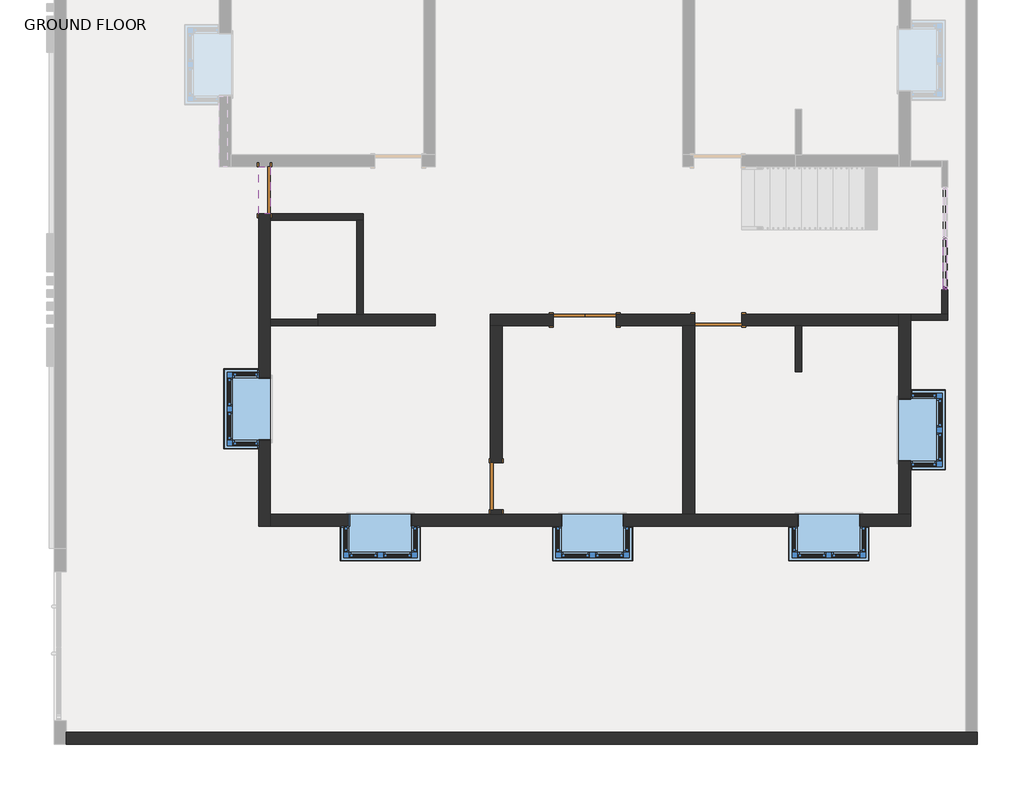
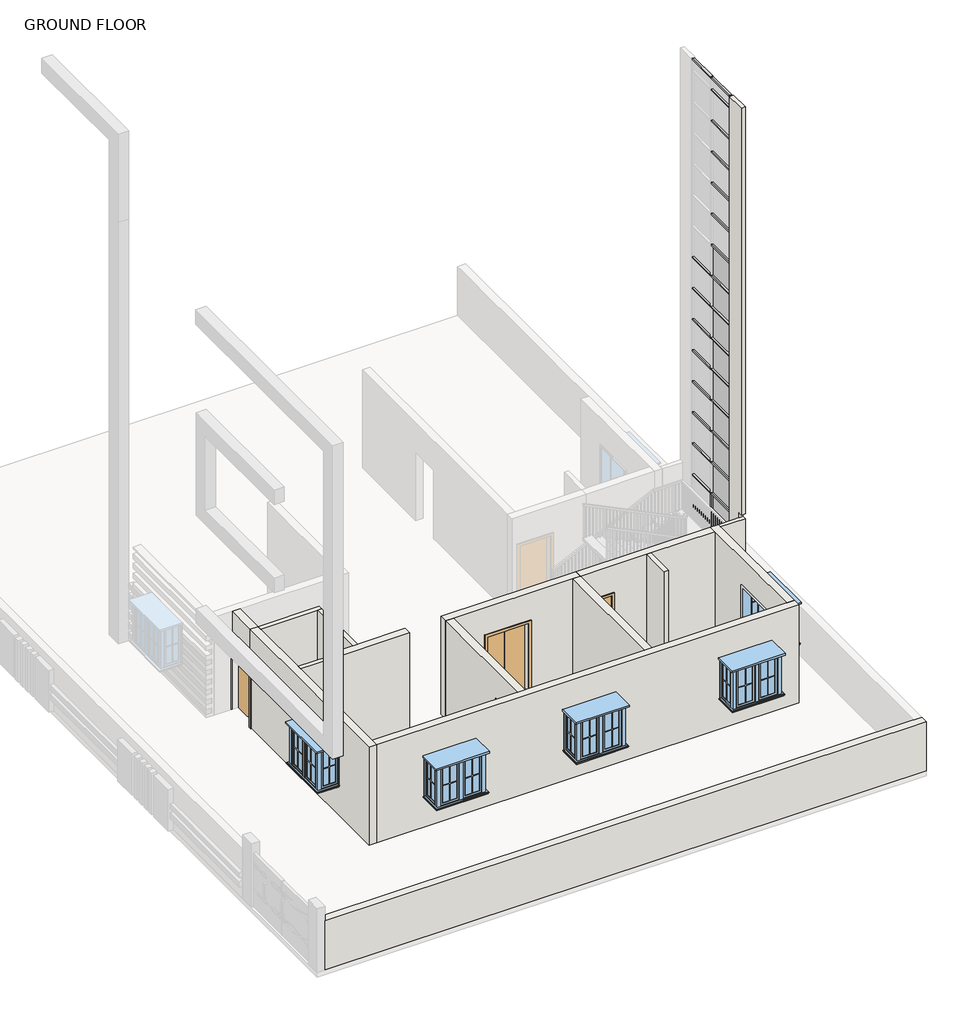
# One storey, part 1 of 5: 66 members, 16 walls, 11 plates, 5 windows, 4 doors.
"""IFC4 building model written with IfcOpenShell, lengths in millimetres."""

from ifc_helpers import new_model, si_unit, frame, origin, origin_with_axes, place, context, project, spatial, polyline, outline, extrude, faceted_brep, transform, mapped, element, save
from components import door_double_flush_panel_4_x7_7c704b5a, door_a90ba1ad, door_0ca8825f, member_c65a811d, member_51048147, member_2967a2d8, member_1ede677d, member_eea045b6, member_e7145701, member_32999801, member_18929904, system_panel_glazed_7f04015b, window_bay_casement_box_90_degree_angle_4_x4_x2_07b705a1

model = new_model("IFC4")

# Units and contexts
model_context = context("Model", 3, world=origin())
ifc_project = project(units=[si_unit("LENGTHUNIT", "METRE", prefix="MILLI")], contexts=[model_context])

# Site, building, storey
site = spatial("IfcSite", under=ifc_project)
building = spatial("IfcBuilding", under=site)
storey = spatial("IfcBuildingStorey", under=building, Name="GROUND FLOOR", Elevation=0.0)

# Doors
placement = place(None, origin())
door_double_flush_panel_4_x7_shape = door_double_flush_panel_4_x7_7c704b5a(model_context)
element("IfcDoor", 1, ObjectType="Door-Double-Flush_Panel : 4'x7'", at=placement, inside=storey, context=model_context, shape_type="MappedRepresentation", body=[
    mapped(door_double_flush_panel_4_x7_shape, transform((78.2584916, -2751.066654, 0.0), x_axis=(1.0, 0.0, 0.0), y_axis=(0.0, 1.0, 0.0), z_axis=(0.0, 0.0, 1.0))),
])
door_shape = door_a90ba1ad(model_context)
element("IfcDoor", 2, ObjectType="Single-Flush : 36\" x 84\"", at=placement, inside=storey, context=model_context, shape_type="MappedRepresentation", body=[
    mapped(door_shape, transform((-1636.2415084, -5976.866654, 0.0), x_axis=(0.0, -1.0, 0.0), y_axis=(1.0, 0.0, 0.0), z_axis=(0.0, 0.0, 1.0))),
])
door_2_shape = door_0ca8825f(model_context)
element("IfcDoor", 3, ObjectType="Single-Flush : 36\" x 84\"", at=placement, inside=storey, context=model_context, shape_type="MappedRepresentation", body=[
    mapped(door_2_shape, transform((2669.0584916, -2751.066654, 0.0), x_axis=(-1.0, 0.0, 0.0), y_axis=(0.0, -1.0, 0.0), z_axis=(0.0, 0.0, 1.0))),
])
element("IfcDoor", 4, ObjectType="Single-Flush : 36\" x 84\"", at=placement, inside=storey, context=model_context, shape_type="MappedRepresentation", body=[
    mapped(door_2_shape, transform((-6132.0415084, -236.466654, 0.0), x_axis=(0.0, -1.0, 0.0), y_axis=(1.0, 0.0, 0.0), z_axis=(0.0, 0.0, 1.0))),
])

# Members
member_shape = member_c65a811d(model_context)
element("IfcMember", 5, ObjectType="Rectangular Mullion : 1.5\" x 2.5\" rectangular", at=placement, inside=storey, context=model_context, shape_type="MappedRepresentation", body=[
    mapped(member_shape, transform((7067.5550459, -1147.0566543, 15849.6), x_axis=(0.0, 0.0, 1.0), y_axis=(-1.0, 0.0, 0.0), z_axis=(0.0, -1.0, 0.0))),
])
element("IfcMember", 6, ObjectType="Rectangular Mullion : 1.5\" x 2.5\" rectangular", at=placement, inside=storey, context=model_context, shape_type="MappedRepresentation", body=[
    mapped(member_shape, transform((7067.5550459, -2112.2566543, 15849.6), x_axis=(0.0, 0.0, 1.0), y_axis=(-1.0, 0.0, 0.0), z_axis=(0.0, -1.0, 0.0))),
])
element("IfcMember", 7, ObjectType="Rectangular Mullion : 1.5\" x 2.5\" rectangular", at=placement, inside=storey, context=model_context, shape_type="MappedRepresentation", body=[
    mapped(member_shape, transform((7067.5550459, -1185.1566543, 0.0), x_axis=(0.0, 0.0, -1.0), y_axis=(-1.0, 0.0, 0.0), z_axis=(0.0, 1.0, 0.0))),
])
member_2_shape = member_51048147(model_context)
element("IfcMember", 8, ObjectType="Rectangular Mullion : 1.5\" x 2.5\" rectangular", at=placement, inside=storey, context=model_context, shape_type="MappedRepresentation", body=[
    mapped(member_2_shape, transform((7067.5550459, -1147.0566543, 984.25), x_axis=(0.0, 0.0, 1.0), y_axis=(-1.0, 0.0, 0.0), z_axis=(0.0, -1.0, 0.0))),
])
element("IfcMember", 9, ObjectType="Rectangular Mullion : 1.5\" x 2.5\" rectangular", at=placement, inside=storey, context=model_context, shape_type="MappedRepresentation", body=[
    mapped(member_2_shape, transform((7067.5550459, -2112.2566543, 984.25), x_axis=(0.0, 0.0, 1.0), y_axis=(-1.0, 0.0, 0.0), z_axis=(0.0, -1.0, 0.0))),
])
element("IfcMember", 10, ObjectType="Rectangular Mullion : 1.5\" x 2.5\" rectangular", at=placement, inside=storey, context=model_context, shape_type="MappedRepresentation", body=[
    mapped(member_2_shape, transform((7067.5550459, -1147.0566543, 1949.45), x_axis=(0.0, 0.0, 1.0), y_axis=(-1.0, 0.0, 0.0), z_axis=(0.0, -1.0, 0.0))),
])
element("IfcMember", 11, ObjectType="Rectangular Mullion : 1.5\" x 2.5\" rectangular", at=placement, inside=storey, context=model_context, shape_type="MappedRepresentation", body=[
    mapped(member_2_shape, transform((7067.5550459, -2112.2566543, 1949.45), x_axis=(0.0, 0.0, 1.0), y_axis=(-1.0, 0.0, 0.0), z_axis=(0.0, -1.0, 0.0))),
])
element("IfcMember", 12, ObjectType="Rectangular Mullion : 1.5\" x 2.5\" rectangular", at=placement, inside=storey, context=model_context, shape_type="MappedRepresentation", body=[
    mapped(member_2_shape, transform((7067.5550459, -1147.0566543, 2914.65), x_axis=(0.0, 0.0, 1.0), y_axis=(-1.0, 0.0, 0.0), z_axis=(0.0, -1.0, 0.0))),
])
element("IfcMember", 13, ObjectType="Rectangular Mullion : 1.5\" x 2.5\" rectangular", at=placement, inside=storey, context=model_context, shape_type="MappedRepresentation", body=[
    mapped(member_2_shape, transform((7067.5550459, -2112.2566543, 2914.65), x_axis=(0.0, 0.0, 1.0), y_axis=(-1.0, 0.0, 0.0), z_axis=(0.0, -1.0, 0.0))),
])
element("IfcMember", 14, ObjectType="Rectangular Mullion : 1.5\" x 2.5\" rectangular", at=placement, inside=storey, context=model_context, shape_type="MappedRepresentation", body=[
    mapped(member_2_shape, transform((7067.5550459, -1147.0566543, 3879.85), x_axis=(0.0, 0.0, 1.0), y_axis=(-1.0, 0.0, 0.0), z_axis=(0.0, -1.0, 0.0))),
])
element("IfcMember", 15, ObjectType="Rectangular Mullion : 1.5\" x 2.5\" rectangular", at=placement, inside=storey, context=model_context, shape_type="MappedRepresentation", body=[
    mapped(member_2_shape, transform((7067.5550459, -2112.2566543, 3879.85), x_axis=(0.0, 0.0, 1.0), y_axis=(-1.0, 0.0, 0.0), z_axis=(0.0, -1.0, 0.0))),
])
element("IfcMember", 16, ObjectType="Rectangular Mullion : 1.5\" x 2.5\" rectangular", at=placement, inside=storey, context=model_context, shape_type="MappedRepresentation", body=[
    mapped(member_2_shape, transform((7067.5550459, -1147.0566543, 4845.05), x_axis=(0.0, 0.0, 1.0), y_axis=(-1.0, 0.0, 0.0), z_axis=(0.0, -1.0, 0.0))),
])
element("IfcMember", 17, ObjectType="Rectangular Mullion : 1.5\" x 2.5\" rectangular", at=placement, inside=storey, context=model_context, shape_type="MappedRepresentation", body=[
    mapped(member_2_shape, transform((7067.5550459, -2112.2566543, 4845.05), x_axis=(0.0, 0.0, 1.0), y_axis=(-1.0, 0.0, 0.0), z_axis=(0.0, -1.0, 0.0))),
])
element("IfcMember", 18, ObjectType="Rectangular Mullion : 1.5\" x 2.5\" rectangular", at=placement, inside=storey, context=model_context, shape_type="MappedRepresentation", body=[
    mapped(member_2_shape, transform((7067.5550459, -1147.0566543, 5810.25), x_axis=(0.0, 0.0, 1.0), y_axis=(-1.0, 0.0, 0.0), z_axis=(0.0, -1.0, 0.0))),
])
element("IfcMember", 19, ObjectType="Rectangular Mullion : 1.5\" x 2.5\" rectangular", at=placement, inside=storey, context=model_context, shape_type="MappedRepresentation", body=[
    mapped(member_2_shape, transform((7067.5550459, -2112.2566543, 5810.25), x_axis=(0.0, 0.0, 1.0), y_axis=(-1.0, 0.0, 0.0), z_axis=(0.0, -1.0, 0.0))),
])
element("IfcMember", 20, ObjectType="Rectangular Mullion : 1.5\" x 2.5\" rectangular", at=placement, inside=storey, context=model_context, shape_type="MappedRepresentation", body=[
    mapped(member_2_shape, transform((7067.5550459, -1147.0566543, 6775.45), x_axis=(0.0, 0.0, 1.0), y_axis=(-1.0, 0.0, 0.0), z_axis=(0.0, -1.0, 0.0))),
])
element("IfcMember", 21, ObjectType="Rectangular Mullion : 1.5\" x 2.5\" rectangular", at=placement, inside=storey, context=model_context, shape_type="MappedRepresentation", body=[
    mapped(member_2_shape, transform((7067.5550459, -2112.2566543, 6775.45), x_axis=(0.0, 0.0, 1.0), y_axis=(-1.0, 0.0, 0.0), z_axis=(0.0, -1.0, 0.0))),
])
element("IfcMember", 22, ObjectType="Rectangular Mullion : 1.5\" x 2.5\" rectangular", at=placement, inside=storey, context=model_context, shape_type="MappedRepresentation", body=[
    mapped(member_2_shape, transform((7067.5550459, -1147.0566543, 7740.65), x_axis=(0.0, 0.0, 1.0), y_axis=(-1.0, 0.0, 0.0), z_axis=(0.0, -1.0, 0.0))),
])
element("IfcMember", 23, ObjectType="Rectangular Mullion : 1.5\" x 2.5\" rectangular", at=placement, inside=storey, context=model_context, shape_type="MappedRepresentation", body=[
    mapped(member_2_shape, transform((7067.5550459, -2112.2566543, 7740.65), x_axis=(0.0, 0.0, 1.0), y_axis=(-1.0, 0.0, 0.0), z_axis=(0.0, -1.0, 0.0))),
])
element("IfcMember", 24, ObjectType="Rectangular Mullion : 1.5\" x 2.5\" rectangular", at=placement, inside=storey, context=model_context, shape_type="MappedRepresentation", body=[
    mapped(member_2_shape, transform((7067.5550459, -1147.0566543, 8705.85), x_axis=(0.0, 0.0, 1.0), y_axis=(-1.0, 0.0, 0.0), z_axis=(0.0, -1.0, 0.0))),
])
element("IfcMember", 25, ObjectType="Rectangular Mullion : 1.5\" x 2.5\" rectangular", at=placement, inside=storey, context=model_context, shape_type="MappedRepresentation", body=[
    mapped(member_2_shape, transform((7067.5550459, -2112.2566543, 8705.85), x_axis=(0.0, 0.0, 1.0), y_axis=(-1.0, 0.0, 0.0), z_axis=(0.0, -1.0, 0.0))),
])
element("IfcMember", 26, ObjectType="Rectangular Mullion : 1.5\" x 2.5\" rectangular", at=placement, inside=storey, context=model_context, shape_type="MappedRepresentation", body=[
    mapped(member_2_shape, transform((7067.5550459, -1147.0566543, 9671.05), x_axis=(0.0, 0.0, 1.0), y_axis=(-1.0, 0.0, 0.0), z_axis=(0.0, -1.0, 0.0))),
])
element("IfcMember", 27, ObjectType="Rectangular Mullion : 1.5\" x 2.5\" rectangular", at=placement, inside=storey, context=model_context, shape_type="MappedRepresentation", body=[
    mapped(member_2_shape, transform((7067.5550459, -2112.2566543, 9671.05), x_axis=(0.0, 0.0, 1.0), y_axis=(-1.0, 0.0, 0.0), z_axis=(0.0, -1.0, 0.0))),
])
element("IfcMember", 28, ObjectType="Rectangular Mullion : 1.5\" x 2.5\" rectangular", at=placement, inside=storey, context=model_context, shape_type="MappedRepresentation", body=[
    mapped(member_2_shape, transform((7067.5550459, -2112.2566543, 10636.25), x_axis=(0.0, 0.0, 1.0), y_axis=(-1.0, 0.0, 0.0), z_axis=(0.0, -1.0, 0.0))),
])
element("IfcMember", 29, ObjectType="Rectangular Mullion : 1.5\" x 2.5\" rectangular", at=placement, inside=storey, context=model_context, shape_type="MappedRepresentation", body=[
    mapped(member_2_shape, transform((7067.5550459, -2112.2566543, 11601.45), x_axis=(0.0, 0.0, 1.0), y_axis=(-1.0, 0.0, 0.0), z_axis=(0.0, -1.0, 0.0))),
])
element("IfcMember", 30, ObjectType="Rectangular Mullion : 1.5\" x 2.5\" rectangular", at=placement, inside=storey, context=model_context, shape_type="MappedRepresentation", body=[
    mapped(member_2_shape, transform((7067.5550459, -2112.2566543, 12566.65), x_axis=(0.0, 0.0, 1.0), y_axis=(-1.0, 0.0, 0.0), z_axis=(0.0, -1.0, 0.0))),
])
element("IfcMember", 31, ObjectType="Rectangular Mullion : 1.5\" x 2.5\" rectangular", at=placement, inside=storey, context=model_context, shape_type="MappedRepresentation", body=[
    mapped(member_2_shape, transform((7067.5550459, -2112.2566543, 13531.85), x_axis=(0.0, 0.0, 1.0), y_axis=(-1.0, 0.0, 0.0), z_axis=(0.0, -1.0, 0.0))),
])
element("IfcMember", 32, ObjectType="Rectangular Mullion : 1.5\" x 2.5\" rectangular", at=placement, inside=storey, context=model_context, shape_type="MappedRepresentation", body=[
    mapped(member_2_shape, transform((7067.5550459, -2112.2566543, 14497.05), x_axis=(0.0, 0.0, 1.0), y_axis=(-1.0, 0.0, 0.0), z_axis=(0.0, -1.0, 0.0))),
])
element("IfcMember", 33, ObjectType="Rectangular Mullion : 1.5\" x 2.5\" rectangular", at=placement, inside=storey, context=model_context, shape_type="MappedRepresentation", body=[
    mapped(member_2_shape, transform((7067.5550459, -2112.2566543, 15462.25), x_axis=(0.0, 0.0, 1.0), y_axis=(-1.0, 0.0, 0.0), z_axis=(0.0, -1.0, 0.0))),
])
member_3_shape = member_2967a2d8(model_context)
element("IfcMember", 34, ObjectType="Rectangular Mullion : 1.5\" x 2.5\" rectangular", at=placement, inside=storey, context=model_context, shape_type="MappedRepresentation", body=[
    mapped(member_3_shape, transform((7067.5550459, -1166.1066543, 0.0), x_axis=(0.0, -1.0, 0.0), y_axis=(-1.0, 0.0, 0.0), z_axis=(0.0, 0.0, -1.0))),
])
element("IfcMember", 35, ObjectType="Rectangular Mullion : 1.5\" x 2.5\" rectangular", at=placement, inside=storey, context=model_context, shape_type="MappedRepresentation", body=[
    mapped(member_3_shape, transform((7067.5550459, -2131.3066543, 0.0), x_axis=(0.0, -1.0, 0.0), y_axis=(-1.0, 0.0, 0.0), z_axis=(0.0, 0.0, -1.0))),
])
member_4_shape = member_1ede677d(model_context)
element("IfcMember", 36, ObjectType="Rectangular Mullion : 1.5\" x 2.5\" rectangular", at=placement, inside=storey, context=model_context, shape_type="MappedRepresentation", body=[
    mapped(member_4_shape, transform((7067.5550459, -1166.1066543, 984.25), x_axis=(0.0, -1.0, 0.0), y_axis=(-1.0, 0.0, 0.0), z_axis=(0.0, 0.0, -1.0))),
])
element("IfcMember", 37, ObjectType="Rectangular Mullion : 1.5\" x 2.5\" rectangular", at=placement, inside=storey, context=model_context, shape_type="MappedRepresentation", body=[
    mapped(member_4_shape, transform((7067.5550459, -1166.1066543, 1949.45), x_axis=(0.0, -1.0, 0.0), y_axis=(-1.0, 0.0, 0.0), z_axis=(0.0, 0.0, -1.0))),
])
element("IfcMember", 38, ObjectType="Rectangular Mullion : 1.5\" x 2.5\" rectangular", at=placement, inside=storey, context=model_context, shape_type="MappedRepresentation", body=[
    mapped(member_4_shape, transform((7067.5550459, -2131.3066543, 984.25), x_axis=(0.0, -1.0, 0.0), y_axis=(-1.0, 0.0, 0.0), z_axis=(0.0, 0.0, -1.0))),
])
element("IfcMember", 39, ObjectType="Rectangular Mullion : 1.5\" x 2.5\" rectangular", at=placement, inside=storey, context=model_context, shape_type="MappedRepresentation", body=[
    mapped(member_4_shape, transform((7067.5550459, -2131.3066543, 1949.45), x_axis=(0.0, -1.0, 0.0), y_axis=(-1.0, 0.0, 0.0), z_axis=(0.0, 0.0, -1.0))),
])
element("IfcMember", 40, ObjectType="Rectangular Mullion : 1.5\" x 2.5\" rectangular", at=placement, inside=storey, context=model_context, shape_type="MappedRepresentation", body=[
    mapped(member_4_shape, transform((7067.5550459, -2131.3066543, 2914.65), x_axis=(0.0, -1.0, 0.0), y_axis=(-1.0, 0.0, 0.0), z_axis=(0.0, 0.0, -1.0))),
])
element("IfcMember", 41, ObjectType="Rectangular Mullion : 1.5\" x 2.5\" rectangular", at=placement, inside=storey, context=model_context, shape_type="MappedRepresentation", body=[
    mapped(member_4_shape, transform((7067.5550459, -2131.3066543, 3879.85), x_axis=(0.0, -1.0, 0.0), y_axis=(-1.0, 0.0, 0.0), z_axis=(0.0, 0.0, -1.0))),
])
element("IfcMember", 42, ObjectType="Rectangular Mullion : 1.5\" x 2.5\" rectangular", at=placement, inside=storey, context=model_context, shape_type="MappedRepresentation", body=[
    mapped(member_4_shape, transform((7067.5550459, -2131.3066543, 4845.05), x_axis=(0.0, -1.0, 0.0), y_axis=(-1.0, 0.0, 0.0), z_axis=(0.0, 0.0, -1.0))),
])
element("IfcMember", 43, ObjectType="Rectangular Mullion : 1.5\" x 2.5\" rectangular", at=placement, inside=storey, context=model_context, shape_type="MappedRepresentation", body=[
    mapped(member_4_shape, transform((7067.5550459, -2131.3066543, 5810.25), x_axis=(0.0, -1.0, 0.0), y_axis=(-1.0, 0.0, 0.0), z_axis=(0.0, 0.0, -1.0))),
])
element("IfcMember", 44, ObjectType="Rectangular Mullion : 1.5\" x 2.5\" rectangular", at=placement, inside=storey, context=model_context, shape_type="MappedRepresentation", body=[
    mapped(member_4_shape, transform((7067.5550459, -2131.3066543, 6775.45), x_axis=(0.0, -1.0, 0.0), y_axis=(-1.0, 0.0, 0.0), z_axis=(0.0, 0.0, -1.0))),
])
element("IfcMember", 45, ObjectType="Rectangular Mullion : 1.5\" x 2.5\" rectangular", at=placement, inside=storey, context=model_context, shape_type="MappedRepresentation", body=[
    mapped(member_4_shape, transform((7067.5550459, -2131.3066543, 7740.65), x_axis=(0.0, -1.0, 0.0), y_axis=(-1.0, 0.0, 0.0), z_axis=(0.0, 0.0, -1.0))),
])
element("IfcMember", 46, ObjectType="Rectangular Mullion : 1.5\" x 2.5\" rectangular", at=placement, inside=storey, context=model_context, shape_type="MappedRepresentation", body=[
    mapped(member_4_shape, transform((7067.5550459, -2131.3066543, 8705.85), x_axis=(0.0, -1.0, 0.0), y_axis=(-1.0, 0.0, 0.0), z_axis=(0.0, 0.0, -1.0))),
])
element("IfcMember", 47, ObjectType="Rectangular Mullion : 1.5\" x 2.5\" rectangular", at=placement, inside=storey, context=model_context, shape_type="MappedRepresentation", body=[
    mapped(member_4_shape, transform((7067.5550459, -2131.3066543, 9671.05), x_axis=(0.0, -1.0, 0.0), y_axis=(-1.0, 0.0, 0.0), z_axis=(0.0, 0.0, -1.0))),
])
element("IfcMember", 48, ObjectType="Rectangular Mullion : 1.5\" x 2.5\" rectangular", at=placement, inside=storey, context=model_context, shape_type="MappedRepresentation", body=[
    mapped(member_4_shape, transform((7067.5550459, -2131.3066543, 10636.25), x_axis=(0.0, -1.0, 0.0), y_axis=(-1.0, 0.0, 0.0), z_axis=(0.0, 0.0, -1.0))),
])
element("IfcMember", 49, ObjectType="Rectangular Mullion : 1.5\" x 2.5\" rectangular", at=placement, inside=storey, context=model_context, shape_type="MappedRepresentation", body=[
    mapped(member_4_shape, transform((7067.5550459, -2131.3066543, 11601.45), x_axis=(0.0, -1.0, 0.0), y_axis=(-1.0, 0.0, 0.0), z_axis=(0.0, 0.0, -1.0))),
])
element("IfcMember", 50, ObjectType="Rectangular Mullion : 1.5\" x 2.5\" rectangular", at=placement, inside=storey, context=model_context, shape_type="MappedRepresentation", body=[
    mapped(member_4_shape, transform((7067.5550459, -2131.3066543, 12566.65), x_axis=(0.0, -1.0, 0.0), y_axis=(-1.0, 0.0, 0.0), z_axis=(0.0, 0.0, -1.0))),
])
element("IfcMember", 51, ObjectType="Rectangular Mullion : 1.5\" x 2.5\" rectangular", at=placement, inside=storey, context=model_context, shape_type="MappedRepresentation", body=[
    mapped(member_4_shape, transform((7067.5550459, -2131.3066543, 13531.85), x_axis=(0.0, -1.0, 0.0), y_axis=(-1.0, 0.0, 0.0), z_axis=(0.0, 0.0, -1.0))),
])
element("IfcMember", 52, ObjectType="Rectangular Mullion : 1.5\" x 2.5\" rectangular", at=placement, inside=storey, context=model_context, shape_type="MappedRepresentation", body=[
    mapped(member_4_shape, transform((7067.5550459, -2131.3066543, 14497.05), x_axis=(0.0, -1.0, 0.0), y_axis=(-1.0, 0.0, 0.0), z_axis=(0.0, 0.0, -1.0))),
])
member_5_shape = member_eea045b6(model_context)
element("IfcMember", 53, ObjectType="Rectangular Mullion : 1.5\" x 2.5\" rectangular", at=placement, inside=storey, context=model_context, shape_type="MappedRepresentation", body=[
    mapped(member_5_shape, transform((7067.5550459, -2131.3066543, 15462.25), x_axis=(0.0, -1.0, 0.0), y_axis=(-1.0, 0.0, 0.0), z_axis=(0.0, 0.0, -1.0))),
])
member_6_shape = member_e7145701(model_context)
element("IfcMember", 54, ObjectType="Rectangular Mullion : 1.5\" x 2.5\" rectangular", at=placement, inside=storey, context=model_context, shape_type="MappedRepresentation", body=[
    mapped(member_6_shape, transform((7067.5550459, -2163.056654, 0.0), x_axis=(0.0, -1.0, 0.0), y_axis=(-1.0, 0.0, 0.0), z_axis=(0.0, 0.0, -1.0))),
])
member_7_shape = member_32999801(model_context)
element("IfcMember", 55, ObjectType="Rectangular Mullion : 1.5\" x 2.5\" rectangular", at=placement, inside=storey, context=model_context, shape_type="MappedRepresentation", body=[
    mapped(member_7_shape, transform((7067.5550459, -2163.056654, 984.25), x_axis=(0.0, -1.0, 0.0), y_axis=(-1.0, 0.0, 0.0), z_axis=(0.0, 0.0, -1.0))),
])
element("IfcMember", 56, ObjectType="Rectangular Mullion : 1.5\" x 2.5\" rectangular", at=placement, inside=storey, context=model_context, shape_type="MappedRepresentation", body=[
    mapped(member_7_shape, transform((7067.5550459, -2163.056654, 1949.45), x_axis=(0.0, -1.0, 0.0), y_axis=(-1.0, 0.0, 0.0), z_axis=(0.0, 0.0, -1.0))),
])
element("IfcMember", 57, ObjectType="Rectangular Mullion : 1.5\" x 2.5\" rectangular", at=placement, inside=storey, context=model_context, shape_type="MappedRepresentation", body=[
    mapped(member_7_shape, transform((7067.5550459, -2163.056654, 2914.65), x_axis=(0.0, -1.0, 0.0), y_axis=(-1.0, 0.0, 0.0), z_axis=(0.0, 0.0, -1.0))),
])
element("IfcMember", 58, ObjectType="Rectangular Mullion : 1.5\" x 2.5\" rectangular", at=placement, inside=storey, context=model_context, shape_type="MappedRepresentation", body=[
    mapped(member_7_shape, transform((7067.5550459, -2163.056654, 3879.85), x_axis=(0.0, -1.0, 0.0), y_axis=(-1.0, 0.0, 0.0), z_axis=(0.0, 0.0, -1.0))),
])
element("IfcMember", 59, ObjectType="Rectangular Mullion : 1.5\" x 2.5\" rectangular", at=placement, inside=storey, context=model_context, shape_type="MappedRepresentation", body=[
    mapped(member_7_shape, transform((7067.5550459, -2163.056654, 4845.05), x_axis=(0.0, -1.0, 0.0), y_axis=(-1.0, 0.0, 0.0), z_axis=(0.0, 0.0, -1.0))),
])
element("IfcMember", 60, ObjectType="Rectangular Mullion : 1.5\" x 2.5\" rectangular", at=placement, inside=storey, context=model_context, shape_type="MappedRepresentation", body=[
    mapped(member_7_shape, transform((7067.5550459, -2163.056654, 5810.25), x_axis=(0.0, -1.0, 0.0), y_axis=(-1.0, 0.0, 0.0), z_axis=(0.0, 0.0, -1.0))),
])
element("IfcMember", 61, ObjectType="Rectangular Mullion : 1.5\" x 2.5\" rectangular", at=placement, inside=storey, context=model_context, shape_type="MappedRepresentation", body=[
    mapped(member_7_shape, transform((7067.5550459, -2163.056654, 6775.45), x_axis=(0.0, -1.0, 0.0), y_axis=(-1.0, 0.0, 0.0), z_axis=(0.0, 0.0, -1.0))),
])
element("IfcMember", 62, ObjectType="Rectangular Mullion : 1.5\" x 2.5\" rectangular", at=placement, inside=storey, context=model_context, shape_type="MappedRepresentation", body=[
    mapped(member_7_shape, transform((7067.5550459, -2163.056654, 7740.65), x_axis=(0.0, -1.0, 0.0), y_axis=(-1.0, 0.0, 0.0), z_axis=(0.0, 0.0, -1.0))),
])
element("IfcMember", 63, ObjectType="Rectangular Mullion : 1.5\" x 2.5\" rectangular", at=placement, inside=storey, context=model_context, shape_type="MappedRepresentation", body=[
    mapped(member_7_shape, transform((7067.5550459, -2163.056654, 8705.85), x_axis=(0.0, -1.0, 0.0), y_axis=(-1.0, 0.0, 0.0), z_axis=(0.0, 0.0, -1.0))),
])
element("IfcMember", 64, ObjectType="Rectangular Mullion : 1.5\" x 2.5\" rectangular", at=placement, inside=storey, context=model_context, shape_type="MappedRepresentation", body=[
    mapped(member_7_shape, transform((7067.5550459, -2163.056654, 9671.05), x_axis=(0.0, -1.0, 0.0), y_axis=(-1.0, 0.0, 0.0), z_axis=(0.0, 0.0, -1.0))),
])
element("IfcMember", 65, ObjectType="Rectangular Mullion : 1.5\" x 2.5\" rectangular", at=placement, inside=storey, context=model_context, shape_type="MappedRepresentation", body=[
    mapped(member_7_shape, transform((7067.5550459, -2163.056654, 10636.25), x_axis=(0.0, -1.0, 0.0), y_axis=(-1.0, 0.0, 0.0), z_axis=(0.0, 0.0, -1.0))),
])
element("IfcMember", 66, ObjectType="Rectangular Mullion : 1.5\" x 2.5\" rectangular", at=placement, inside=storey, context=model_context, shape_type="MappedRepresentation", body=[
    mapped(member_7_shape, transform((7067.5550459, -2163.056654, 11601.45), x_axis=(0.0, -1.0, 0.0), y_axis=(-1.0, 0.0, 0.0), z_axis=(0.0, 0.0, -1.0))),
])
element("IfcMember", 67, ObjectType="Rectangular Mullion : 1.5\" x 2.5\" rectangular", at=placement, inside=storey, context=model_context, shape_type="MappedRepresentation", body=[
    mapped(member_7_shape, transform((7067.5550459, -2163.056654, 12566.65), x_axis=(0.0, -1.0, 0.0), y_axis=(-1.0, 0.0, 0.0), z_axis=(0.0, 0.0, -1.0))),
])
element("IfcMember", 68, ObjectType="Rectangular Mullion : 1.5\" x 2.5\" rectangular", at=placement, inside=storey, context=model_context, shape_type="MappedRepresentation", body=[
    mapped(member_7_shape, transform((7067.5550459, -2163.056654, 13531.85), x_axis=(0.0, -1.0, 0.0), y_axis=(-1.0, 0.0, 0.0), z_axis=(0.0, 0.0, -1.0))),
])
element("IfcMember", 69, ObjectType="Rectangular Mullion : 1.5\" x 2.5\" rectangular", at=placement, inside=storey, context=model_context, shape_type="MappedRepresentation", body=[
    mapped(member_7_shape, transform((7067.5550459, -2163.056654, 14497.05), x_axis=(0.0, -1.0, 0.0), y_axis=(-1.0, 0.0, 0.0), z_axis=(0.0, 0.0, -1.0))),
])
member_8_shape = member_18929904(model_context)
element("IfcMember", 70, ObjectType="Rectangular Mullion : 1.5\" x 2.5\" rectangular", at=placement, inside=storey, context=model_context, shape_type="MappedRepresentation", body=[
    mapped(member_8_shape, transform((7067.5550459, -2163.056654, 15462.25), x_axis=(0.0, -1.0, 0.0), y_axis=(-1.0, 0.0, 0.0), z_axis=(0.0, 0.0, -1.0))),
])

# Plates
system_panel_glazed_shape = system_panel_glazed_7f04015b(model_context)
element("IfcPlate", 71, ObjectType="System Panel : Glazed", at=placement, inside=storey, context=model_context, shape_type="MappedRepresentation", body=[
    mapped(system_panel_glazed_shape, transform((7067.5550459, -1648.7066543, 38.1), x_axis=(0.0, -1.0, 0.0), y_axis=(1.0, 0.0, 0.0), z_axis=(0.0, 0.0, 1.0))),
])
element("IfcPlate", 72, ObjectType="System Panel : Glazed", at=placement, inside=storey, context=model_context, shape_type="MappedRepresentation", body=[
    mapped(system_panel_glazed_shape, transform((7067.5550459, -1648.7066543, 1003.3), x_axis=(0.0, -1.0, 0.0), y_axis=(1.0, 0.0, 0.0), z_axis=(0.0, 0.0, 1.0))),
])
element("IfcPlate", 73, ObjectType="System Panel : Glazed", at=placement, inside=storey, context=model_context, shape_type="MappedRepresentation", body=[
    mapped(system_panel_glazed_shape, transform((7067.5550459, -1648.7066543, 1968.5), x_axis=(0.0, -1.0, 0.0), y_axis=(1.0, 0.0, 0.0), z_axis=(0.0, 0.0, 1.0))),
])
element("IfcPlate", 74, ObjectType="System Panel : Glazed", at=placement, inside=storey, context=model_context, shape_type="MappedRepresentation", body=[
    mapped(system_panel_glazed_shape, transform((7067.5550459, -1648.7066543, 2933.7), x_axis=(0.0, -1.0, 0.0), y_axis=(1.0, 0.0, 0.0), z_axis=(0.0, 0.0, 1.0))),
])
element("IfcPlate", 75, ObjectType="System Panel : Glazed", at=placement, inside=storey, context=model_context, shape_type="MappedRepresentation", body=[
    mapped(system_panel_glazed_shape, transform((7067.5550459, -1648.7066543, 3898.9), x_axis=(0.0, -1.0, 0.0), y_axis=(1.0, 0.0, 0.0), z_axis=(0.0, 0.0, 1.0))),
])
element("IfcPlate", 76, ObjectType="System Panel : Glazed", at=placement, inside=storey, context=model_context, shape_type="MappedRepresentation", body=[
    mapped(system_panel_glazed_shape, transform((7067.5550459, -1648.7066543, 4864.1), x_axis=(0.0, -1.0, 0.0), y_axis=(1.0, 0.0, 0.0), z_axis=(0.0, 0.0, 1.0))),
])
element("IfcPlate", 77, ObjectType="System Panel : Glazed", at=placement, inside=storey, context=model_context, shape_type="MappedRepresentation", body=[
    mapped(system_panel_glazed_shape, transform((7067.5550459, -1648.7066543, 5829.3), x_axis=(0.0, -1.0, 0.0), y_axis=(1.0, 0.0, 0.0), z_axis=(0.0, 0.0, 1.0))),
])
element("IfcPlate", 78, ObjectType="System Panel : Glazed", at=placement, inside=storey, context=model_context, shape_type="MappedRepresentation", body=[
    mapped(system_panel_glazed_shape, transform((7067.5550459, -1648.7066543, 6794.5), x_axis=(0.0, -1.0, 0.0), y_axis=(1.0, 0.0, 0.0), z_axis=(0.0, 0.0, 1.0))),
])
element("IfcPlate", 79, ObjectType="System Panel : Glazed", at=placement, inside=storey, context=model_context, shape_type="MappedRepresentation", body=[
    mapped(system_panel_glazed_shape, transform((7067.5550459, -1648.7066543, 7759.7), x_axis=(0.0, -1.0, 0.0), y_axis=(1.0, 0.0, 0.0), z_axis=(0.0, 0.0, 1.0))),
])
element("IfcPlate", 80, ObjectType="System Panel : Glazed", at=placement, inside=storey, context=model_context, shape_type="MappedRepresentation", body=[
    mapped(system_panel_glazed_shape, transform((7067.5550459, -1648.7066543, 8724.9), x_axis=(0.0, -1.0, 0.0), y_axis=(1.0, 0.0, 0.0), z_axis=(0.0, 0.0, 1.0))),
])
element("IfcPlate", 81, ObjectType="System Panel : Glazed", at=placement, inside=storey, context=model_context, shape_type="MappedRepresentation", body=[
    mapped(system_panel_glazed_shape, transform((7067.5550459, -1648.7066543, 9690.1), x_axis=(0.0, -1.0, 0.0), y_axis=(1.0, 0.0, 0.0), z_axis=(0.0, 0.0, 1.0))),
])

# Walls
element("IfcWall", 82, ObjectType="4.6\"", at=placement, inside=storey, context=model_context, shape_type="Brep", body=[
    faceted_brep([(6402.8584916, -2753.606654, 0.0), (7125.9750459, -2753.606654, 0.0), (7125.9750459, -2753.606654, 3048.0), (6402.8584916, -2753.606654, 3048.0), (6402.8584916, -2636.766654, 0.0), (6402.8584916, -2636.766654, 3048.0), (7125.9750459, -2636.766654, 3048.0), (7125.9750459, -2636.766654, 0.0), (7009.1350459, -2636.766654, 0.0)], [[[0, 1, 2, 3]], [[4, 5, 6, 7, 8]], [[1, 0, 4, 8, 7]], [[3, 2, 6, 5]], [[0, 3, 5, 4]], [[2, 1, 7, 6]]]),
])
element("IfcWall", 83, ObjectType="4.6\"", at=placement, inside=storey, context=model_context, shape_type="Brep", body=[
    faceted_brep([(7125.9750459, -2636.766654, 0.0), (7125.9750459, -2163.056654, 0.0), (7125.9750459, -2163.056654, 15849.6), (7125.9750459, -2753.606654, 15849.6), (7125.9750459, -2753.606654, 3200.4), (7125.9750459, -2636.766654, 3200.4), (7125.9750459, -2636.766654, 3048.0), (7009.1350459, -2636.766654, 0.0), (7009.1350459, -2636.766654, 3200.4), (7009.1350459, -2753.606654, 3200.4), (7009.1350459, -2753.606654, 6248.4), (7009.1350459, -2753.606654, 6400.8), (7009.1350459, -2753.606654, 9448.8), (7009.1350459, -2753.606654, 9601.2), (7009.1350459, -2753.606654, 12649.2), (7009.1350459, -2753.606654, 12801.6), (7009.1350459, -2753.606654, 15849.6), (7009.1350459, -2639.306654, 15849.6), (7009.1350459, -2163.056654, 15849.6), (7009.1350459, -2163.056654, 0.0)], [[[0, 1, 2, 3, 4, 5, 6]], [[7, 8, 9, 10, 11, 12, 13, 14, 15, 16, 17, 18, 19]], [[1, 0, 7, 19]], [[2, 1, 19, 18]], [[3, 2, 18, 17, 16]], [[4, 9, 8, 5]], [[0, 6, 5, 8, 7]], [[3, 16, 15, 14, 13, 12, 11, 10, 9, 4]]]),
])
element("IfcWall", 84, ObjectType="5\"", at=placement, inside=storey, context=model_context, shape_type="SweptSolid", body=[
    extrude(outline(polyline([(4159.1868368, -3751.826654), (4159.1868368, -2865.366654), (4286.1868368, -2865.366654), (4286.1868368, -3751.826654), (4159.1868368, -3751.826654)])), origin_with_axes(), (0.0, 0.0, 1.0), 3048.0),
])
element("IfcWall", 85, ObjectType="5\"", at=placement, inside=storey, context=model_context, shape_type="Brep", body=[
    faceted_brep([(-6017.7415084, -820.666654, 0.0), (-4341.3415084, -820.666654, 0.0), (-4214.3415084, -820.666654, 0.0), (-4214.3415084, -820.666654, 3048.0), (-4341.3415084, -820.666654, 3048.0), (-6017.7415084, -820.666654, 3048.0), (-6017.7415084, -693.666654, 0.0), (-6017.7415084, -693.666654, 3048.0), (-4214.3415084, -693.666654, 3048.0), (-4214.3415084, -693.666654, 0.0)], [[[0, 1, 2, 3, 4, 5]], [[6, 7, 8, 9]], [[2, 1, 0, 6, 9]], [[5, 4, 3, 8, 7]], [[0, 5, 7, 6]], [[3, 2, 9, 8]]]),
])
element("IfcWall", 86, ObjectType="5\"", at=placement, inside=storey, context=model_context, shape_type="SweptSolid", body=[
    extrude(outline(polyline([(-4341.3415084, -2636.766654), (-4341.3415084, -820.666654), (-4214.3415084, -820.666654), (-4214.3415084, -2636.766654), (-4341.3415084, -2636.766654)])), origin_with_axes(), (0.0, 0.0, 1.0), 3048.0),
])
element("IfcWall", 87, ObjectType="5\"", at=placement, inside=storey, context=model_context, shape_type="SweptSolid", body=[
    extrude(outline(polyline([(-6017.7415084, -2738.366654), (-5103.3415084, -2738.366654), (-5103.3415084, -2865.366654), (-6017.7415084, -2865.366654), (-6017.7415084, -2738.366654)])), origin_with_axes(), (0.0, 0.0, 1.0), 3048.0),
])
element("IfcWall", 88, ObjectType="9\"", at=placement, inside=storey, context=model_context, shape_type="Brep", body=[
    faceted_brep([(-6246.3415084, -693.666654, 0.0), (-6246.3415084, -6751.566654, 0.0), (-6246.3415084, -6751.566654, 3048.0), (-6246.3415084, -693.666654, 3048.0), (-6246.3415084, -693.666654, 2133.6), (-6246.3415084, -3868.666654, 2184.4), (-6246.3415084, -5087.866654, 2184.4), (-6246.3415084, -5087.866654, 914.4), (-6246.3415084, -3868.666654, 914.4), (-6017.7415084, -693.666654, 0.0), (-6017.7415084, -693.666654, 2133.6), (-6017.7415084, -693.666654, 3048.0), (-6017.7415084, -820.666654, 3048.0), (-6017.7415084, -2738.366654, 3048.0), (-6017.7415084, -2865.366654, 3048.0), (-6017.7415084, -6522.966654, 3048.0), (-6017.7415084, -6751.566654, 3048.0), (-6017.7415084, -6751.566654, 0.0), (-6017.7415084, -6522.966654, 0.0), (-6017.7415084, -2865.366654, 0.0), (-6017.7415084, -2738.366654, 0.0), (-6017.7415084, -820.666654, 0.0), (-6017.7415084, -3868.666654, 2184.4), (-6017.7415084, -3868.666654, 914.4), (-6017.7415084, -5087.866654, 914.4), (-6017.7415084, -5087.866654, 2184.4)], [[[0, 1, 2, 3, 4], [5, 6, 7, 8]], [[9, 10, 11, 12, 13, 14, 15, 16, 17, 18, 19, 20, 21], [22, 23, 24, 25]], [[1, 0, 9, 21, 20, 19, 18, 17]], [[3, 2, 16, 15, 14, 13, 12, 11]], [[2, 1, 17, 16]], [[0, 4, 3, 11, 10, 9]], [[23, 22, 5, 8]], [[24, 23, 8, 7]], [[25, 24, 7, 6]], [[22, 25, 6, 5]]]),
])
element("IfcWall", 89, ObjectType="9\"", at=placement, inside=storey, context=model_context, shape_type="Brep", body=[
    faceted_brep([(-2817.3415084, -2636.766654, 0.0), (-4214.3415084, -2636.766654, 0.0), (-4341.3415084, -2636.766654, 0.0), (-5103.3415084, -2636.766654, 0.0), (-5103.3415084, -2636.766654, 3048.0), (-4341.3415084, -2636.766654, 3048.0), (-4214.3415084, -2636.766654, 3048.0), (-2817.3415084, -2636.766654, 3048.0), (-2817.3415084, -2865.366654, 0.0), (-2817.3415084, -2865.366654, 3048.0), (-5103.3415084, -2865.366654, 3048.0), (-5103.3415084, -2865.366654, 0.0), (-5103.3415084, -2738.366654, 0.0), (-5103.3415084, -2738.366654, 3048.0)], [[[0, 1, 2, 3, 4, 5, 6, 7]], [[8, 9, 10, 11]], [[3, 2, 1, 0, 8, 11, 12]], [[4, 3, 12, 11, 10, 13]], [[7, 6, 5, 4, 13, 10, 9]], [[0, 7, 9, 8]]]),
])
element("IfcWall", 90, ObjectType="9\"", at=placement, inside=storey, context=model_context, shape_type="Brep", body=[
    faceted_brep([(2211.8584916, -2865.366654, 3048.0), (1983.2584916, -2865.366654, 3048.0), (-1521.9415084, -2865.366654, 3048.0), (-1750.5415084, -2865.366654, 3048.0), (-1750.5415084, -2865.366654, 0.0), (-1521.9415084, -2865.366654, 0.0), (-531.3415084, -2865.366654, 0.0), (-531.3415084, -2865.366654, 2133.6), (687.8584916, -2865.366654, 2133.6), (687.8584916, -2865.366654, 0.0), (1983.2584916, -2865.366654, 0.0), (2211.8584916, -2865.366654, 0.0), (2211.8584916, -2865.366654, 2133.6), (-1750.5415084, -2636.766654, 3048.0), (2211.8584916, -2636.766654, 3048.0), (2211.8584916, -2636.766654, 2133.6), (2211.8584916, -2636.766654, 0.0), (687.8584916, -2636.766654, 0.0), (687.8584916, -2636.766654, 2133.6), (-531.3415084, -2636.766654, 2133.6), (-531.3415084, -2636.766654, 0.0), (-1750.5415084, -2636.766654, 0.0)], [[[0, 1, 2, 3, 4, 5, 6, 7, 8, 9, 10, 11, 12]], [[13, 14, 15, 16, 17, 18, 19, 20, 21]], [[16, 11, 10, 9, 17]], [[4, 21, 20, 6, 5]], [[3, 2, 1, 0, 14, 13]], [[0, 12, 11, 16, 15, 14]], [[4, 3, 13, 21]], [[8, 18, 17, 9]], [[18, 8, 7, 19]], [[19, 7, 6, 20]]]),
])
element("IfcWall", 91, ObjectType="9\"", at=placement, inside=storey, context=model_context, shape_type="SweptSolid", body=[
    extrude(outline(polyline([(1983.2584916, -6522.966654), (1983.2584916, -2865.366654), (2211.8584916, -2865.366654), (2211.8584916, -6522.966654), (1983.2584916, -6522.966654)])), origin_with_axes(), (0.0, 0.0, 1.0), 3048.0),
])
element("IfcWall", 92, ObjectType="9\"", at=placement, inside=storey, context=model_context, shape_type="Brep", body=[
    faceted_brep([(-6017.7415084, -6751.566654, 0.0), (6402.8584916, -6751.566654, 0.0), (6402.8584916, -6751.566654, 3048.0), (-6017.7415084, -6751.566654, 3048.0), (-378.9415084, -6751.566654, 2184.4), (840.2584916, -6751.566654, 2184.4), (840.2584916, -6751.566654, 914.4), (-378.9415084, -6751.566654, 914.4), (4205.7584916, -6751.566654, 2184.4), (5424.9584916, -6751.566654, 2184.4), (5424.9584916, -6751.566654, 914.4), (4205.7584916, -6751.566654, 914.4), (-4493.7415084, -6751.566654, 2184.4), (-3274.5415084, -6751.566654, 2184.4), (-3274.5415084, -6751.566654, 914.4), (-4493.7415084, -6751.566654, 914.4), (-6017.7415084, -6522.966654, 0.0), (-6017.7415084, -6522.966654, 3048.0), (-1750.5415084, -6522.966654, 3048.0), (-1521.9415084, -6522.966654, 3048.0), (1983.2584916, -6522.966654, 3048.0), (2211.8584916, -6522.966654, 3048.0), (6174.2584916, -6522.966654, 3048.0), (6402.8584916, -6522.966654, 3048.0), (6402.8584916, -6522.966654, 0.0), (6174.2584916, -6522.966654, 0.0), (2211.8584916, -6522.966654, 0.0), (1983.2584916, -6522.966654, 0.0), (-1521.9415084, -6522.966654, 0.0), (-1750.5415084, -6522.966654, 0.0), (-378.9415084, -6522.966654, 2184.4), (-378.9415084, -6522.966654, 914.4), (840.2584916, -6522.966654, 914.4), (840.2584916, -6522.966654, 2184.4), (4205.7584916, -6522.966654, 2184.4), (4205.7584916, -6522.966654, 914.4), (5424.9584916, -6522.966654, 914.4), (5424.9584916, -6522.966654, 2184.4), (-4493.7415084, -6522.966654, 2184.4), (-4493.7415084, -6522.966654, 914.4), (-3274.5415084, -6522.966654, 914.4), (-3274.5415084, -6522.966654, 2184.4)], [[[0, 1, 2, 3], [4, 5, 6, 7], [8, 9, 10, 11], [12, 13, 14, 15]], [[16, 17, 18, 19, 20, 21, 22, 23, 24, 25, 26, 27, 28, 29], [30, 31, 32, 33], [34, 35, 36, 37], [38, 39, 40, 41]], [[1, 0, 16, 29, 28, 27, 26, 25, 24]], [[3, 2, 23, 22, 21, 20, 19, 18, 17]], [[2, 1, 24, 23]], [[0, 3, 17, 16]], [[31, 30, 4, 7]], [[32, 31, 7, 6]], [[33, 32, 6, 5]], [[30, 33, 5, 4]], [[35, 34, 8, 11]], [[36, 35, 11, 10]], [[37, 36, 10, 9]], [[34, 37, 9, 8]], [[39, 38, 12, 15]], [[40, 39, 15, 14]], [[41, 40, 14, 13]], [[38, 41, 13, 12]]]),
])
element("IfcWall", 93, ObjectType="9\"", at=placement, inside=storey, context=model_context, shape_type="Brep", body=[
    faceted_brep([(6402.8584916, -6522.966654, 0.0), (6402.8584916, -2753.606654, 0.0), (6402.8584916, -2636.766654, 0.0), (6402.8584916, -2636.766654, 3048.0), (6402.8584916, -2753.606654, 3048.0), (6402.8584916, -6522.966654, 3048.0), (6402.8584916, -5494.266654, 2184.4), (6402.8584916, -4275.066654, 2184.4), (6402.8584916, -4275.066654, 914.4), (6402.8584916, -5494.266654, 914.4), (6174.2584916, -6522.966654, 0.0), (6174.2584916, -6522.966654, 3048.0), (6174.2584916, -2865.366654, 3048.0), (6174.2584916, -2636.766654, 3048.0), (6174.2584916, -2636.766654, 0.0), (6174.2584916, -2865.366654, 0.0), (6174.2584916, -5494.266654, 2184.4), (6174.2584916, -5494.266654, 914.4), (6174.2584916, -4275.066654, 914.4), (6174.2584916, -4275.066654, 2184.4)], [[[0, 1, 2, 3, 4, 5], [6, 7, 8, 9]], [[10, 11, 12, 13, 14, 15], [16, 17, 18, 19]], [[2, 1, 0, 10, 15, 14]], [[5, 4, 3, 13, 12, 11]], [[0, 5, 11, 10]], [[3, 2, 14, 13]], [[17, 16, 6, 9]], [[18, 17, 9, 8]], [[19, 18, 8, 7]], [[16, 19, 7, 6]]]),
])
element("IfcWall", 94, ObjectType="9\"", at=placement, inside=storey, context=model_context, shape_type="Brep", body=[
    faceted_brep([(2211.8584916, -2636.766654, 3048.0), (6174.2584916, -2636.766654, 3048.0), (6174.2584916, -2636.766654, 0.0), (3126.2584916, -2636.766654, 0.0), (3126.2584916, -2636.766654, 2133.6), (2211.8584916, -2636.766654, 2133.6), (6174.2584916, -2865.366654, 3048.0), (4286.1868368, -2865.366654, 3048.0), (4159.1868368, -2865.366654, 3048.0), (2211.8584916, -2865.366654, 3048.0), (2211.8584916, -2865.366654, 2133.6), (3126.2584916, -2865.366654, 2133.6), (3126.2584916, -2865.366654, 0.0), (4159.1868368, -2865.366654, 0.0), (4286.1868368, -2865.366654, 0.0), (6174.2584916, -2865.366654, 0.0)], [[[0, 1, 2, 3, 4, 5]], [[6, 7, 8, 9, 10, 11, 12, 13, 14, 15]], [[2, 15, 14, 13, 12, 3]], [[1, 0, 9, 8, 7, 6]], [[2, 1, 6, 15]], [[9, 0, 5, 10]], [[4, 11, 10, 5]], [[11, 4, 3, 12]]]),
])
element("IfcWall", 95, ObjectType="9\"", at=placement, inside=storey, context=model_context, shape_type="SweptSolid", body=[
    extrude(outline(polyline([(-6434.066654, 2133.6), (-6434.066654, 0.0), (-6522.966654, 0.0), (-6522.966654, 3048.0), (-2865.366654, 3048.0), (-2865.366654, 0.0), (-5519.666654, 0.0), (-5519.666654, 2133.6), (-6434.066654, 2133.6)])), frame((-1750.5415084, 0.0, 0.0), z_axis=(1.0, 0.0, 0.0), x_axis=(0.0, 1.0, 0.0)), (0.0, 0.0, 1.0), 228.6),
])
element("IfcWall", 96, ObjectType="9\"", at=placement, inside=storey, context=model_context, shape_type="SweptSolid", body=[
    extrude(outline(polyline([(-6017.7415084, 220.733346), (-6017.7415084, -693.666654), (-6246.3415084, -693.666654), (-6246.3415084, 220.733346), (-6017.7415084, 220.733346)])), frame((0.0, 0.0, 2133.6), z_axis=(0.0, 0.0, 1.0), x_axis=(1.0, 0.0, 0.0)), (0.0, 0.0, 1.0), 914.4),
])
element("IfcWall", 97, ObjectType="9\"", at=placement, inside=storey, context=model_context, shape_type="Brep", body=[
    faceted_brep([(-9980.1415084, -10980.666654, 0.0), (7698.2584916, -10980.666654, 0.0), (7698.2584916, -10980.666654, 1524.0), (-9980.1415084, -10980.666654, 1524.0), (-9980.1415084, -10752.066654, 0.0), (-9980.1415084, -10752.066654, 1524.0), (7469.6584916, -10752.066654, 1524.0), (7698.2584916, -10752.066654, 1524.0), (7698.2584916, -10752.066654, 0.0), (7469.6584916, -10752.066654, 0.0)], [[[0, 1, 2, 3]], [[4, 5, 6, 7, 8, 9]], [[1, 0, 4, 9, 8]], [[3, 2, 7, 6, 5]], [[0, 3, 5, 4]], [[2, 1, 8, 7]]]),
])

# Windows
window_bay_casement_box_90_degree_angle_4_x4_x2_shape = window_bay_casement_box_90_degree_angle_4_x4_x2_07b705a1(model_context)
element("IfcWindow", 98, ObjectType="Window-Bay-Casement-Box-90_Degree_Angle : 4'X4'X2'", at=placement, inside=storey, context=model_context, shape_type="MappedRepresentation", body=[
    mapped(window_bay_casement_box_90_degree_angle_4_x4_x2_shape, transform((-6132.0415084, -4478.266654, 304.8), x_axis=(0.0, 1.0, 0.0), y_axis=(-1.0, 0.0, 0.0), z_axis=(0.0, 0.0, 1.0))),
])
element("IfcWindow", 99, ObjectType="Window-Bay-Casement-Box-90_Degree_Angle : 4'X4'X2'", at=placement, inside=storey, context=model_context, shape_type="MappedRepresentation", body=[
    mapped(window_bay_casement_box_90_degree_angle_4_x4_x2_shape, transform((6288.5584916, -4884.666654, 304.8), x_axis=(0.0, -1.0, 0.0), y_axis=(1.0, 0.0, 0.0), z_axis=(0.0, 0.0, 1.0))),
])
element("IfcWindow", 100, ObjectType="Window-Bay-Casement-Box-90_Degree_Angle : 4'X4'X2'", at=placement, inside=storey, context=model_context, shape_type="MappedRepresentation", body=[
    mapped(window_bay_casement_box_90_degree_angle_4_x4_x2_shape, transform((230.6584916, -6637.266654, 304.8), x_axis=(-1.0, 0.0, 0.0), y_axis=(0.0, -1.0, 0.0), z_axis=(0.0, 0.0, 1.0))),
])
element("IfcWindow", 101, ObjectType="Window-Bay-Casement-Box-90_Degree_Angle : 4'X4'X2'", at=placement, inside=storey, context=model_context, shape_type="MappedRepresentation", body=[
    mapped(window_bay_casement_box_90_degree_angle_4_x4_x2_shape, transform((4815.3584916, -6637.266654, 304.8), x_axis=(-1.0, 0.0, 0.0), y_axis=(0.0, -1.0, 0.0), z_axis=(0.0, 0.0, 1.0))),
])
element("IfcWindow", 102, ObjectType="Window-Bay-Casement-Box-90_Degree_Angle : 4'X4'X2'", at=placement, inside=storey, context=model_context, shape_type="MappedRepresentation", body=[
    mapped(window_bay_casement_box_90_degree_angle_4_x4_x2_shape, transform((-3884.1415084, -6637.266654, 304.8), x_axis=(-1.0, 0.0, 0.0), y_axis=(0.0, -1.0, 0.0), z_axis=(0.0, 0.0, 1.0))),
])

save(model, "model.ifc")

# Revit data of these elements
# Type "Door-Double-Flush_Panel : 4'x7'"
#   Type Mark = "9"
#   Construction Type Id = "DOOR"
#   Assembly Code = "C1020"
#   Analytic Construction = "Wooden"
#   Thickness = 0' - 2"
#   Thermal Resistance (R) = 2.5876 (h·ft²·°F)/BTU
#   Swing Angle [instance default] = 90.00°
#   Panel Width = 2' - 0"
#   Heat Transfer Coefficient (U) = 0.3865 BTU/(h·ft²·°F)
#   Height = 7' - 0"
#   Trim Projection Ext = 0' - 1"
#   Trim Projection Int = 0' - 1"
#   Trim Width = 0' - 3"
#   Width = 4' - 0"
#   Define Thermal Properties by = 1
#   Panel Material = Wood - Birch - Solid Stained Light Low Gloss
#   Trim Material = Paint - Sienna
#   Visual Light Transmittance = 0
#   Solar Heat Gain Coefficient = 0
#   Function = (empty or 0)
#   Wall Closure = (empty or 0)
# Type "Single-Flush : 36\" x 84\""
#   Type Mark = "1"
#   Construction Type Id = "MDOOR"
#   Assembly Code = "C1020"
#   Analytic Construction = "Metal"
#   Thickness = 0' - 2"
#   Heat Transfer Coefficient (U) = 0.651978 BTU/(h·ft²·°F)
#   Height = 7' - 0"
#   Trim Projection Ext = 0' - 1"
#   Trim Projection Int = 0' - 1"
#   Trim Width = 0' - 3"
#   Width = 3' - 0"
#   Define Thermal Properties by = 1
#   Define Thermal Properties by = 1
#   Door Material = Door - Panel
#   Frame Material = Door - Frame
#   Visual Light Transmittance = 0
#   Solar Heat Gain Coefficient = 0
#   Function = (empty or 0)
#   Wall Closure = (empty or 0)
# Type "Rectangular Mullion : 1.5\" x 2.5\" rectangular"
#   built-in parameter 1007304 = 0.208333 (stored number, unit not read)
#   built-in parameter 1007301 = 0.0625 (stored number, unit not read)
#   built-in parameter 1007300 = 0.0625 (stored number, unit not read)
# Type "System Panel : Glazed"
#   Construction Type Id = "GSP4R"
#   Analytic Construction = "1/8 in Pilkington single glazing"
#   Visual Light Transmittance = 0.9
#   Solar Heat Gain Coefficient = 0.86
#   Heat Transfer Coefficient (U) = 1.18115 BTU/(h·ft²·°F)
#   Define Thermal Properties by = 1
# Type "4.6\""
#   Assembly Code = "B2010"
#   Layers, outside or top first: 0' - 4 77/128" no material (function 1)
# Type "5\""
#   Assembly Code = "B2010"
#   Layers, outside or top first: 0' - 5" no material (function 1)
# Type "9\""
#   Assembly Code = "B2010"
#   Layers, outside or top first: 0' - 9" "WALL 1" (function 1)
# Type "Window-Bay-Casement-Box-90_Degree_Angle : 4'X4'X2'"
#   Type Mark = "20"
#   Fire Rating = "0.5h"
#   Assembly Code = "B2020100"
#   Analytic Construction = "1/8 in Pilkington single glazing"
#   Width = 4' - 0"
#   Wall Thickness [instance default] = 0' - 6"
#   Visual Light Transmittance = 0.9
#   Trim Width = 4' - 8"
#   Trim Height = 4' - 0"
#   Thermal Resistance (R) = 1.5394 (h·ft²·°F)/BTU
#   Solar Heat Gain Coefficient = 0.86
#   Rough Width = 4' - 0 1/2"
#   Rough Height = 4' - 0 1/2"
#   Height 1 = 4' - 2"
#   Height = 4' - 0"
#   Heat Transfer Coefficient (U) = 0.6496 BTU/(h·ft²·°F)
#   Depth = 2' - 0"
#   Default Sill Height = 2' - 0"
#   Muntin Visibility = yes
#   Interior Trim Visibility [instance default] = yes
#   Exterior Trim Visibility [instance default] = yes
#   Muntin Pattern = Muntin Pattern_2x2 : Muntin Pattern_2x2
#   Interior Trim Material = Wood - Stained
#   Exterior Trim Material = Clad - White
#   Exterior Trim = element 423684
#   Interior Trim = Trim-Window-Interior-Flat : Picture Frame
#   Interior Frame Material = Wood - Stained
#   Glass Panel Material = Glass
#   Exterior Frame Material = Clad - White
#   Wall Closure = (empty or 0)
# Element 1 (IfcDoor, "Door-Double-Flush_Panel : 4'x7'")
#   Swing Angle = 90.00°
#   Phase Created = New Construction
#   Materials on its faces: "Paint - Sienna", "Wood - Birch - Solid Stained Light Low Gloss"
# Elements 2, 3, 4 (IfcDoor, "Single-Flush : 36\" x 84\"")
#   Phase Created = New Construction
#   Materials on its faces: "Door - Frame", "Door - Panel"
# Elements 5, 6, 7, 8, 9, 10, 11, 12, 13, 14, 15, 16, 17, 18, 19, 20, 21, 22, 23, 24, 25, 26, 27, 28, 29, 30, 31, 32, 33, 34, 35, 36, 37, 38, 39, 40, 41, 42, 43, 44, 45, 46, 47, 48, 49, 50, 51, 52, 53, 54, 55, 56, 57, 58, 59, 60, 61, 62, 63, 64, 65, 66, 67, 68, 69, 70 (IfcMember, "Rectangular Mullion : 1.5\" x 2.5\" rectangular")
#   Phase Created = New Construction
#   Materials on its faces: "Aluminum"
# Elements 71, 72, 73, 74, 75, 76, 77, 78, 79, 80, 81 (IfcPlate, "System Panel : Glazed")
#   Phase Created = New Construction
#   Materials on its faces: "Glass"
# Element 82 (IfcWall, "4.6\"")
#   Top Offset = -0' - 6"
#   Base Offset = 0' - 0"
#   wall height = 10' - 0"
#   Phase Created = New Construction
#   Base Constraint = GROUND FLOOR
#   Top Constraint = FIRST FLOOR
#   Materials on its faces: "Default Wall", "WALL 2", "WALL 3"
# Element 83 (IfcWall, "4.6\"")
#   Top Offset = -0' - 6"
#   Base Offset = 0' - 0"
#   wall height = 52' - 0"
#   Phase Created = New Construction
#   Base Constraint = GROUND FLOOR
#   Top Constraint = ROOF
#   Materials on its faces: "Default Wall", "WALL 3", "WALL 1"
# Elements 84, 85, 86, 87 (IfcWall, "5\"")
#   Top Offset = -0' - 6"
#   Base Offset = 0' - 0"
#   wall height = 10' - 0"
#   Phase Created = New Construction
#   Base Constraint = GROUND FLOOR
#   Top Constraint = FIRST FLOOR
#   Materials on its faces: "Default Wall"
# Element 88 (IfcWall, "9\"")
#   Top Offset = -0' - 6"
#   Base Offset = 0' - 0"
#   wall height = 10' - 0"
#   Phase Created = New Construction
#   Base Constraint = GROUND FLOOR
#   Top Constraint = FIRST FLOOR
#   Materials on its faces: "WALL 1", "WALL 2", "Default Wall"
# Elements 89, 90, 91, 94, 95 (IfcWall, "9\"")
#   Top Offset = -0' - 6"
#   Base Offset = 0' - 0"
#   wall height = 10' - 0"
#   Phase Created = New Construction
#   Base Constraint = GROUND FLOOR
#   Top Constraint = FIRST FLOOR
#   Materials on its faces: "WALL 1"
# Elements 92, 93, 96 (IfcWall, "9\"")
#   Top Offset = -0' - 6"
#   Base Offset = 0' - 0"
#   wall height = 10' - 0"
#   Phase Created = New Construction
#   Base Constraint = GROUND FLOOR
#   Top Constraint = FIRST FLOOR
#   Materials on its faces: "WALL 1", "WALL 2"
# Element 97 (IfcWall, "9\"")
#   Top Offset = -0' - 6"
#   Base Offset = 0' - 0"
#   Unconnected Height = 5' - 0"
#   wall height = 5' - 0"
#   Phase Created = New Construction
#   Base Constraint = GROUND FLOOR
#   Materials on its faces: "WALL 4", "WALL 1"
# Element 98 (IfcWindow, "Window-Bay-Casement-Box-90_Degree_Angle : 4'X4'X2'")
#   Mark = "6"
#   Phase Created = New Construction
#   Materials on its faces: "Clad - White", "Wood - Stained", "Glass"
# Element 99 (IfcWindow, "Window-Bay-Casement-Box-90_Degree_Angle : 4'X4'X2'")
#   Mark = "7"
#   Phase Created = New Construction
#   Materials on its faces: "Clad - White", "Wood - Stained", "Glass"
# Element 100 (IfcWindow, "Window-Bay-Casement-Box-90_Degree_Angle : 4'X4'X2'")
#   Mark = "12"
#   Phase Created = New Construction
#   Materials on its faces: "Clad - White", "Wood - Stained", "Glass"
# Element 101 (IfcWindow, "Window-Bay-Casement-Box-90_Degree_Angle : 4'X4'X2'")
#   Mark = "13"
#   Phase Created = New Construction
#   Materials on its faces: "Clad - White", "Wood - Stained", "Glass"
# Element 102 (IfcWindow, "Window-Bay-Casement-Box-90_Degree_Angle : 4'X4'X2'")
#   Mark = "14"
#   Phase Created = New Construction
#   Materials on its faces: "Clad - White", "Wood - Stained", "Glass"
# Materials
#   "Wood - Birch - Solid Stained Light Low Gloss": class "Wood", colour RGB 210 159 95, transparency 0, Cost = 0
#   "Paint - Sienna": colour RGB 118 70 51, transparency 0, Cost = 0
#   "Door - Panel": class "Wood", colour RGB 210 159 95, transparency 0, Cost = 0
#   "Door - Frame": colour RGB 118 70 51, transparency 0, Cost = 0
#   "WALL 1": class "Generic", colour RGB 233 224 215, transparency 0, Cost = 0
#   "Wood - Stained": class "Wood", colour RGB 224 178 126, transparency 0, Cost = 0
#   "Clad - White": class "Wood", colour RGB 242 242 238, transparency 0, Cost = 0
#   "Glass": class "Glass", colour RGB 0 128 192, transparency 0.75, Description = "Soda Lime Glass", Cost = 0
#   "Aluminum": class "Metal", colour RGB 247 247 247, transparency 0, Description = "Aluminum 6061", Cost = 0
#   "Default Wall": colour RGB 128 128 128, transparency 0, Cost = 0
#   "WALL 2": class "Generic", colour RGB 52 58 64, transparency 0, Cost = 0
#   "WALL 3": class "Generic", colour RGB 240 237 232, transparency 0, Cost = 0
#   "WALL 4": class "Generic", colour RGB 32 32 32, transparency 0, Cost = 0
